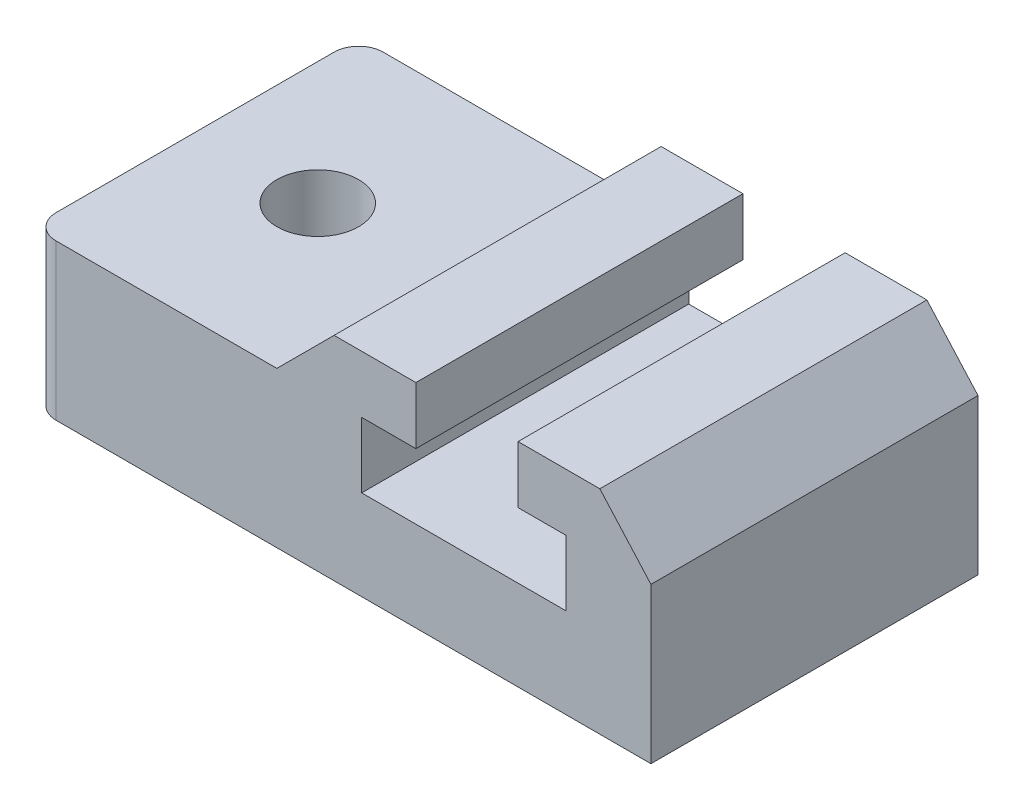
ISO-10303-21;
HEADER;
FILE_DESCRIPTION(('STEP AP214'),'2;1');
FILE_NAME('part.step','',(''),(''),'','','');
FILE_SCHEMA(('AUTOMOTIVE_DESIGN { 1 0 10303 214 1 1 1 1 }'));
ENDSEC;
DATA;
#1=APPLICATION_CONTEXT('core data for automotive mechanical design processes');
#2=APPLICATION_PROTOCOL_DEFINITION('international standard','automotive_design',2000,#1);
#3=PRODUCT_CONTEXT('',#1,'mechanical');
#4=PRODUCT('Part','Part','',(#3));
#5=PRODUCT_RELATED_PRODUCT_CATEGORY('part','',(#4));
#6=PRODUCT_DEFINITION_FORMATION('','',#4);
#7=PRODUCT_DEFINITION_CONTEXT('part definition',#1,'design');
#8=PRODUCT_DEFINITION('design','',#6,#7);
#9=PRODUCT_DEFINITION_SHAPE('','',#8);
#10=(LENGTH_UNIT() NAMED_UNIT(*) SI_UNIT(.MILLI.,.METRE.));
#11=(NAMED_UNIT(*) PLANE_ANGLE_UNIT() SI_UNIT($,.RADIAN.));
#12=(NAMED_UNIT(*) SI_UNIT($,.STERADIAN.) SOLID_ANGLE_UNIT());
#13=UNCERTAINTY_MEASURE_WITH_UNIT(LENGTH_MEASURE(1.E-05),#10,'distance_accuracy_value','');
#14=(GEOMETRIC_REPRESENTATION_CONTEXT(3) GLOBAL_UNCERTAINTY_ASSIGNED_CONTEXT((#13)) GLOBAL_UNIT_ASSIGNED_CONTEXT((#10,
#11,#12)) REPRESENTATION_CONTEXT('',''));
#15=CARTESIAN_POINT('',(0.,0.,0.));
#16=DIRECTION('',(0.,0.,1.));
#17=DIRECTION('',(1.,0.,0.));
#18=AXIS2_PLACEMENT_3D('',#15,#16,#17);
#19=CARTESIAN_POINT('',(0.,0.,80.));
#20=DIRECTION('',(0.,-1.,0.));
#21=DIRECTION('',(0.,0.,-1.));
#22=AXIS2_PLACEMENT_3D('',#19,#20,#21);
#23=PLANE('',#22);
#24=DIRECTION('',(0.,0.,1.));
#25=VECTOR('',#24,1.);
#26=CARTESIAN_POINT('',(-7.50000000000004,0.,6.));
#27=LINE('',#26,#25);
#28=CARTESIAN_POINT('',(-7.50000000000004,0.,61.0777233158545));
#29=VERTEX_POINT('',#28);
#30=CARTESIAN_POINT('',(-7.50000000000004,0.,74.));
#31=VERTEX_POINT('',#30);
#32=EDGE_CURVE('E308',#29,#31,#27,.T.);
#33=ORIENTED_EDGE('',*,*,#32,.F.);
#34=DIRECTION('',(-1.,0.,0.));
#35=VECTOR('',#34,1.);
#36=CARTESIAN_POINT('',(30.5,0.,61.0777233158545));
#37=LINE('',#36,#35);
#38=CARTESIAN_POINT('',(30.5,0.,61.0777233158545));
#39=VERTEX_POINT('',#38);
#40=EDGE_CURVE('E402',#39,#29,#37,.T.);
#41=ORIENTED_EDGE('',*,*,#40,.F.);
#42=DIRECTION('',(0.,0.,1.));
#43=VECTOR('',#42,1.);
#44=CARTESIAN_POINT('',(30.5,0.,0.));
#45=LINE('',#44,#43);
#46=CARTESIAN_POINT('',(30.5,0.,46.));
#47=VERTEX_POINT('',#46);
#48=EDGE_CURVE('E401',#47,#39,#45,.T.);
#49=ORIENTED_EDGE('',*,*,#48,.F.);
#50=CARTESIAN_POINT('',(22.5,0.,40.));
#51=DIRECTION('',(0.,1.,0.));
#52=DIRECTION('',(0.,0.,1.));
#53=AXIS2_PLACEMENT_3D('',#50,#51,#52);
#54=CIRCLE('',#53,10.);
#55=CARTESIAN_POINT('',(30.5,0.,34.));
#56=VERTEX_POINT('',#55);
#57=EDGE_CURVE('E290',#47,#56,#54,.T.);
#58=ORIENTED_EDGE('',*,*,#57,.T.);
#59=CARTESIAN_POINT('',(30.5,0.,18.2));
#60=VERTEX_POINT('',#59);
#61=EDGE_CURVE('E63',#60,#56,#45,.T.);
#62=ORIENTED_EDGE('',*,*,#61,.F.);
#63=DIRECTION('',(-1.,0.,0.));
#64=VECTOR('',#63,1.);
#65=CARTESIAN_POINT('',(30.5,0.,18.2));
#66=LINE('',#65,#64);
#67=CARTESIAN_POINT('',(-7.50000000000004,0.,18.2));
#68=VERTEX_POINT('',#67);
#69=EDGE_CURVE('E299',#60,#68,#66,.T.);
#70=ORIENTED_EDGE('',*,*,#69,.T.);
#71=CARTESIAN_POINT('',(-7.50000000000004,0.,6.));
#72=VERTEX_POINT('',#71);
#73=EDGE_CURVE('E306',#72,#68,#27,.T.);
#74=ORIENTED_EDGE('',*,*,#73,.F.);
#75=CARTESIAN_POINT('',(-1.50000000000004,0.,6.00000000000001));
#76=DIRECTION('',(0.,1.,0.));
#77=DIRECTION('',(0.,0.,1.));
#78=AXIS2_PLACEMENT_3D('',#75,#76,#77);
#79=CIRCLE('',#78,6.);
#80=CARTESIAN_POINT('',(-1.50000000000004,0.,0.));
#81=VERTEX_POINT('',#80);
#82=EDGE_CURVE('E304',#81,#72,#79,.T.);
#83=ORIENTED_EDGE('',*,*,#82,.F.);
#84=DIRECTION('',(-1.,0.,0.));
#85=VECTOR('',#84,1.);
#86=CARTESIAN_POINT('',(0.,0.,0.));
#87=LINE('',#86,#85);
#88=CARTESIAN_POINT('',(144.,0.,0.));
#89=VERTEX_POINT('',#88);
#90=EDGE_CURVE('E194',#89,#81,#87,.T.);
#91=ORIENTED_EDGE('',*,*,#90,.F.);
#92=DIRECTION('',(0.,0.,-1.));
#93=VECTOR('',#92,1.);
#94=CARTESIAN_POINT('',(144.,0.,80.));
#95=LINE('',#94,#93);
#96=CARTESIAN_POINT('',(144.,0.,80.));
#97=VERTEX_POINT('',#96);
#98=EDGE_CURVE('E251',#97,#89,#95,.T.);
#99=ORIENTED_EDGE('',*,*,#98,.F.);
#100=DIRECTION('',(-1.,0.,0.));
#101=VECTOR('',#100,1.);
#102=CARTESIAN_POINT('',(0.,0.,80.));
#103=LINE('',#102,#101);
#104=CARTESIAN_POINT('',(-1.50000000000004,0.,80.));
#105=VERTEX_POINT('',#104);
#106=EDGE_CURVE('E130',#97,#105,#103,.T.);
#107=ORIENTED_EDGE('',*,*,#106,.T.);
#108=CARTESIAN_POINT('',(-1.50000000000004,0.,74.));
#109=DIRECTION('',(0.,1.,0.));
#110=DIRECTION('',(0.,0.,1.));
#111=AXIS2_PLACEMENT_3D('',#108,#109,#110);
#112=CIRCLE('',#111,6.00000000000001);
#113=EDGE_CURVE('E313',#31,#105,#112,.T.);
#114=ORIENTED_EDGE('',*,*,#113,.F.);
#115=EDGE_LOOP('',(#33,#41,#49,#58,#62,#70,#74,#83,#91,#99,#107,#114));
#116=FACE_BOUND('',#115,.T.);
#117=ADVANCED_FACE('F50',(#116),#23,.T.);
#118=CARTESIAN_POINT('',(-7.50000000000004,0.,6.));
#119=DIRECTION('',(-1.,0.,0.));
#120=DIRECTION('',(0.,0.,1.));
#121=AXIS2_PLACEMENT_3D('',#118,#119,#120);
#122=PLANE('',#121);
#123=ORIENTED_EDGE('',*,*,#73,.T.);
#124=DIRECTION('',(0.,0.888265617173928,-0.459330157236188));
#125=VECTOR('',#124,1.);
#126=CARTESIAN_POINT('',(-7.50000000000004,7.42573077799279,14.3600876810915));
#127=LINE('',#126,#125);
#128=CARTESIAN_POINT('',(-7.50000000000004,11.9897349209895,12.));
#129=VERTEX_POINT('',#128);
#130=EDGE_CURVE('E398',#68,#129,#127,.T.);
#131=ORIENTED_EDGE('',*,*,#130,.T.);
#132=DIRECTION('',(0.,0.,1.));
#133=VECTOR('',#132,1.);
#134=CARTESIAN_POINT('',(-7.50000000000004,11.9897349209895,0.));
#135=LINE('',#134,#133);
#136=CARTESIAN_POINT('',(-7.50000000000004,11.9897349209895,68.));
#137=VERTEX_POINT('',#136);
#138=EDGE_CURVE('E404',#129,#137,#135,.T.);
#139=ORIENTED_EDGE('',*,*,#138,.T.);
#140=DIRECTION('',(0.,-0.866025403784439,-0.5));
#141=VECTOR('',#140,1.);
#142=CARTESIAN_POINT('',(-7.50000000000004,-26.4474299984236,45.8082924868908));
#143=LINE('',#142,#141);
#144=EDGE_CURVE('E412',#137,#29,#143,.T.);
#145=ORIENTED_EDGE('',*,*,#144,.T.);
#146=ORIENTED_EDGE('',*,*,#32,.T.);
#147=DIRECTION('',(0.,1.,0.));
#148=VECTOR('',#147,1.);
#149=CARTESIAN_POINT('',(-7.50000000000004,0.,74.));
#150=LINE('',#149,#148);
#151=CARTESIAN_POINT('',(-7.50000000000004,38.,74.));
#152=VERTEX_POINT('',#151);
#153=EDGE_CURVE('E191',#31,#152,#150,.T.);
#154=ORIENTED_EDGE('',*,*,#153,.T.);
#155=DIRECTION('',(0.,0.,1.));
#156=VECTOR('',#155,1.);
#157=CARTESIAN_POINT('',(-7.50000000000004,38.,6.));
#158=LINE('',#157,#156);
#159=CARTESIAN_POINT('',(-7.50000000000004,38.,6.));
#160=VERTEX_POINT('',#159);
#161=EDGE_CURVE('E294',#160,#152,#158,.T.);
#162=ORIENTED_EDGE('',*,*,#161,.F.);
#163=DIRECTION('',(0.,1.,0.));
#164=VECTOR('',#163,1.);
#165=CARTESIAN_POINT('',(-7.50000000000004,0.,6.));
#166=LINE('',#165,#164);
#167=EDGE_CURVE('E311',#72,#160,#166,.T.);
#168=ORIENTED_EDGE('',*,*,#167,.F.);
#169=EDGE_LOOP('',(#123,#131,#139,#145,#146,#154,#162,#168));
#170=FACE_BOUND('',#169,.T.);
#171=ADVANCED_FACE('F368',(#170),#122,.T.);
#172=CARTESIAN_POINT('',(22.5,0.,40.));
#173=DIRECTION('',(0.,1.,0.));
#174=DIRECTION('',(0.,0.,1.));
#175=AXIS2_PLACEMENT_3D('',#172,#173,#174);
#176=CYLINDRICAL_SURFACE('',#175,10.);
#177=CARTESIAN_POINT('',(22.5,38.,40.));
#178=DIRECTION('',(0.,1.,0.));
#179=DIRECTION('',(0.,0.,1.));
#180=AXIS2_PLACEMENT_3D('',#177,#178,#179);
#181=CIRCLE('',#180,10.);
#182=CARTESIAN_POINT('',(22.5,38.,50.));
#183=VERTEX_POINT('',#182);
#184=EDGE_CURVE('E292',#183,#183,#181,.T.);
#185=ORIENTED_EDGE('',*,*,#184,.T.);
#186=EDGE_LOOP('',(#185));
#187=FACE_BOUND('',#186,.T.);
#188=DIRECTION('',(0.,1.,0.));
#189=VECTOR('',#188,1.);
#190=CARTESIAN_POINT('',(30.5,0.,46.));
#191=LINE('',#190,#189);
#192=CARTESIAN_POINT('',(30.5,11.9897349209895,46.));
#193=VERTEX_POINT('',#192);
#194=EDGE_CURVE('E11',#193,#47,#191,.F.);
#195=ORIENTED_EDGE('',*,*,#194,.F.);
#196=CARTESIAN_POINT('',(22.5,11.9897349209895,40.));
#197=DIRECTION('',(0.,-1.,0.));
#198=DIRECTION('',(0.,0.,-1.));
#199=AXIS2_PLACEMENT_3D('',#196,#197,#198);
#200=CIRCLE('',#199,10.);
#201=CARTESIAN_POINT('',(30.5,11.9897349209895,34.));
#202=VERTEX_POINT('',#201);
#203=EDGE_CURVE('E53',#202,#193,#200,.F.);
#204=ORIENTED_EDGE('',*,*,#203,.F.);
#205=DIRECTION('',(0.,1.,0.));
#206=VECTOR('',#205,1.);
#207=CARTESIAN_POINT('',(30.5,0.,34.));
#208=LINE('',#207,#206);
#209=EDGE_CURVE('E254',#56,#202,#208,.T.);
#210=ORIENTED_EDGE('',*,*,#209,.F.);
#211=ORIENTED_EDGE('',*,*,#57,.F.);
#212=EDGE_LOOP('',(#195,#204,#210,#211));
#213=FACE_BOUND('',#212,.T.);
#214=ADVANCED_FACE('F284',(#187,#213),#176,.F.);
#215=CARTESIAN_POINT('',(144.,0.,80.));
#216=DIRECTION('',(1.,0.,0.));
#217=DIRECTION('',(0.,0.,-1.));
#218=AXIS2_PLACEMENT_3D('',#215,#216,#217);
#219=PLANE('',#218);
#220=DIRECTION('',(0.,-1.,0.));
#221=VECTOR('',#220,1.);
#222=CARTESIAN_POINT('',(144.,0.,0.));
#223=LINE('',#222,#221);
#224=CARTESIAN_POINT('',(144.,38.,0.));
#225=VERTEX_POINT('',#224);
#226=EDGE_CURVE('E197',#225,#89,#223,.T.);
#227=ORIENTED_EDGE('',*,*,#226,.F.);
#228=DIRECTION('',(0.,0.,-1.));
#229=VECTOR('',#228,1.);
#230=CARTESIAN_POINT('',(144.,38.,80.));
#231=LINE('',#230,#229);
#232=CARTESIAN_POINT('',(144.,38.,80.));
#233=VERTEX_POINT('',#232);
#234=EDGE_CURVE('E253',#233,#225,#231,.T.);
#235=ORIENTED_EDGE('',*,*,#234,.F.);
#236=DIRECTION('',(0.,-1.,0.));
#237=VECTOR('',#236,1.);
#238=CARTESIAN_POINT('',(144.,0.,80.));
#239=LINE('',#238,#237);
#240=EDGE_CURVE('E324',#233,#97,#239,.T.);
#241=ORIENTED_EDGE('',*,*,#240,.T.);
#242=ORIENTED_EDGE('',*,*,#98,.T.);
#243=EDGE_LOOP('',(#227,#235,#241,#242));
#244=FACE_BOUND('',#243,.T.);
#245=ADVANCED_FACE('F428',(#244),#219,.T.);
#246=CARTESIAN_POINT('',(99.0035486160397,88.3960255500355,80.));
#247=DIRECTION('',(0.745937661625914,0.666015769308853,0.));
#248=DIRECTION('',(-0.666015769308853,0.745937661625914,0.));
#249=AXIS2_PLACEMENT_3D('',#246,#247,#248);
#250=PLANE('',#249);
#251=DIRECTION('',(0.666015769308853,-0.745937661625914,0.));
#252=VECTOR('',#251,1.);
#253=CARTESIAN_POINT('',(99.0035486160397,88.3960255500355,0.));
#254=LINE('',#253,#252);
#255=CARTESIAN_POINT('',(131.5,52.,0.));
#256=VERTEX_POINT('',#255);
#257=EDGE_CURVE('E199',#256,#225,#254,.T.);
#258=ORIENTED_EDGE('',*,*,#257,.F.);
#259=DIRECTION('',(0.,0.,-1.));
#260=VECTOR('',#259,1.);
#261=CARTESIAN_POINT('',(131.5,52.,80.));
#262=LINE('',#261,#260);
#263=CARTESIAN_POINT('',(131.5,52.,80.));
#264=VERTEX_POINT('',#263);
#265=EDGE_CURVE('E246',#264,#256,#262,.T.);
#266=ORIENTED_EDGE('',*,*,#265,.F.);
#267=DIRECTION('',(0.666015769308853,-0.745937661625914,0.));
#268=VECTOR('',#267,1.);
#269=CARTESIAN_POINT('',(99.0035486160397,88.3960255500355,80.));
#270=LINE('',#269,#268);
#271=EDGE_CURVE('E327',#264,#233,#270,.T.);
#272=ORIENTED_EDGE('',*,*,#271,.T.);
#273=ORIENTED_EDGE('',*,*,#234,.T.);
#274=EDGE_LOOP('',(#258,#266,#272,#273));
#275=FACE_BOUND('',#274,.T.);
#276=ADVANCED_FACE('F435',(#275),#250,.T.);
#277=CARTESIAN_POINT('',(0.,52.,80.));
#278=DIRECTION('',(0.,1.,0.));
#279=DIRECTION('',(0.,0.,1.));
#280=AXIS2_PLACEMENT_3D('',#277,#278,#279);
#281=PLANE('',#280);
#282=DIRECTION('',(1.,0.,0.));
#283=VECTOR('',#282,1.);
#284=CARTESIAN_POINT('',(0.,52.,0.));
#285=LINE('',#284,#283);
#286=CARTESIAN_POINT('',(111.5,52.,0.));
#287=VERTEX_POINT('',#286);
#288=EDGE_CURVE('E201',#287,#256,#285,.T.);
#289=ORIENTED_EDGE('',*,*,#288,.F.);
#290=DIRECTION('',(0.,0.,-1.));
#291=VECTOR('',#290,1.);
#292=CARTESIAN_POINT('',(111.5,52.,80.));
#293=LINE('',#292,#291);
#294=CARTESIAN_POINT('',(111.5,52.,80.));
#295=VERTEX_POINT('',#294);
#296=EDGE_CURVE('E250',#295,#287,#293,.T.);
#297=ORIENTED_EDGE('',*,*,#296,.F.);
#298=DIRECTION('',(1.,0.,0.));
#299=VECTOR('',#298,1.);
#300=CARTESIAN_POINT('',(0.,52.,80.));
#301=LINE('',#300,#299);
#302=EDGE_CURVE('E332',#295,#264,#301,.T.);
#303=ORIENTED_EDGE('',*,*,#302,.T.);
#304=ORIENTED_EDGE('',*,*,#265,.T.);
#305=EDGE_LOOP('',(#289,#297,#303,#304));
#306=FACE_BOUND('',#305,.T.);
#307=ADVANCED_FACE('F436',(#306),#281,.T.);
#308=CARTESIAN_POINT('',(111.5,0.,80.));
#309=DIRECTION('',(1.,0.,0.));
#310=DIRECTION('',(0.,0.,-1.));
#311=AXIS2_PLACEMENT_3D('',#308,#309,#310);
#312=PLANE('',#311);
#313=DIRECTION('',(0.,-1.,0.));
#314=VECTOR('',#313,1.);
#315=CARTESIAN_POINT('',(111.5,0.,0.));
#316=LINE('',#315,#314);
#317=CARTESIAN_POINT('',(111.5,38.,0.));
#318=VERTEX_POINT('',#317);
#319=EDGE_CURVE('E206',#287,#318,#316,.T.);
#320=ORIENTED_EDGE('',*,*,#319,.T.);
#321=DIRECTION('',(0.,0.,-1.));
#322=VECTOR('',#321,1.);
#323=CARTESIAN_POINT('',(111.5,38.,80.));
#324=LINE('',#323,#322);
#325=CARTESIAN_POINT('',(111.5,38.,80.));
#326=VERTEX_POINT('',#325);
#327=EDGE_CURVE('E242',#326,#318,#324,.T.);
#328=ORIENTED_EDGE('',*,*,#327,.F.);
#329=DIRECTION('',(0.,-1.,0.));
#330=VECTOR('',#329,1.);
#331=CARTESIAN_POINT('',(111.5,0.,80.));
#332=LINE('',#331,#330);
#333=EDGE_CURVE('E331',#295,#326,#332,.T.);
#334=ORIENTED_EDGE('',*,*,#333,.F.);
#335=ORIENTED_EDGE('',*,*,#296,.T.);
#336=EDGE_LOOP('',(#320,#328,#334,#335));
#337=FACE_BOUND('',#336,.T.);
#338=ADVANCED_FACE('F442',(#337),#312,.F.);
#339=CARTESIAN_POINT('',(0.,38.,80.));
#340=DIRECTION('',(0.,1.,0.));
#341=DIRECTION('',(0.,0.,1.));
#342=AXIS2_PLACEMENT_3D('',#339,#340,#341);
#343=PLANE('',#342);
#344=DIRECTION('',(1.,0.,0.));
#345=VECTOR('',#344,1.);
#346=CARTESIAN_POINT('',(0.,38.,0.));
#347=LINE('',#346,#345);
#348=CARTESIAN_POINT('',(123.25,38.,0.));
#349=VERTEX_POINT('',#348);
#350=EDGE_CURVE('E208',#318,#349,#347,.T.);
#351=ORIENTED_EDGE('',*,*,#350,.T.);
#352=DIRECTION('',(0.,0.,-1.));
#353=VECTOR('',#352,1.);
#354=CARTESIAN_POINT('',(123.25,38.,80.));
#355=LINE('',#354,#353);
#356=CARTESIAN_POINT('',(123.25,38.,80.));
#357=VERTEX_POINT('',#356);
#358=EDGE_CURVE('E243',#357,#349,#355,.T.);
#359=ORIENTED_EDGE('',*,*,#358,.F.);
#360=DIRECTION('',(1.,0.,0.));
#361=VECTOR('',#360,1.);
#362=CARTESIAN_POINT('',(0.,38.,80.));
#363=LINE('',#362,#361);
#364=EDGE_CURVE('E338',#326,#357,#363,.T.);
#365=ORIENTED_EDGE('',*,*,#364,.F.);
#366=ORIENTED_EDGE('',*,*,#327,.T.);
#367=EDGE_LOOP('',(#351,#359,#365,#366));
#368=FACE_BOUND('',#367,.T.);
#369=ADVANCED_FACE('F450',(#368),#343,.F.);
#370=CARTESIAN_POINT('',(123.25,0.,80.));
#371=DIRECTION('',(1.,0.,0.));
#372=DIRECTION('',(0.,0.,-1.));
#373=AXIS2_PLACEMENT_3D('',#370,#371,#372);
#374=PLANE('',#373);
#375=DIRECTION('',(0.,-1.,0.));
#376=VECTOR('',#375,1.);
#377=CARTESIAN_POINT('',(123.25,0.,0.));
#378=LINE('',#377,#376);
#379=CARTESIAN_POINT('',(123.25,22.,0.));
#380=VERTEX_POINT('',#379);
#381=EDGE_CURVE('E209',#349,#380,#378,.T.);
#382=ORIENTED_EDGE('',*,*,#381,.T.);
#383=DIRECTION('',(0.,0.,-1.));
#384=VECTOR('',#383,1.);
#385=CARTESIAN_POINT('',(123.25,22.,80.));
#386=LINE('',#385,#384);
#387=CARTESIAN_POINT('',(123.25,22.,80.));
#388=VERTEX_POINT('',#387);
#389=EDGE_CURVE('E236',#388,#380,#386,.T.);
#390=ORIENTED_EDGE('',*,*,#389,.F.);
#391=DIRECTION('',(0.,-1.,0.));
#392=VECTOR('',#391,1.);
#393=CARTESIAN_POINT('',(123.25,0.,80.));
#394=LINE('',#393,#392);
#395=EDGE_CURVE('E336',#357,#388,#394,.T.);
#396=ORIENTED_EDGE('',*,*,#395,.F.);
#397=ORIENTED_EDGE('',*,*,#358,.T.);
#398=EDGE_LOOP('',(#382,#390,#396,#397));
#399=FACE_BOUND('',#398,.T.);
#400=ADVANCED_FACE('F452',(#399),#374,.F.);
#401=CARTESIAN_POINT('',(0.,22.,80.));
#402=DIRECTION('',(0.,-1.,0.));
#403=DIRECTION('',(0.,0.,-1.));
#404=AXIS2_PLACEMENT_3D('',#401,#402,#403);
#405=PLANE('',#404);
#406=DIRECTION('',(-1.,0.,0.));
#407=VECTOR('',#406,1.);
#408=CARTESIAN_POINT('',(0.,22.,0.));
#409=LINE('',#408,#407);
#410=CARTESIAN_POINT('',(73.25,22.,0.));
#411=VERTEX_POINT('',#410);
#412=EDGE_CURVE('E215',#380,#411,#409,.T.);
#413=ORIENTED_EDGE('',*,*,#412,.T.);
#414=DIRECTION('',(0.,0.,-1.));
#415=VECTOR('',#414,1.);
#416=CARTESIAN_POINT('',(73.25,22.,80.));
#417=LINE('',#416,#415);
#418=CARTESIAN_POINT('',(73.25,22.,80.));
#419=VERTEX_POINT('',#418);
#420=EDGE_CURVE('E233',#419,#411,#417,.T.);
#421=ORIENTED_EDGE('',*,*,#420,.F.);
#422=DIRECTION('',(-1.,0.,0.));
#423=VECTOR('',#422,1.);
#424=CARTESIAN_POINT('',(0.,22.,80.));
#425=LINE('',#424,#423);
#426=EDGE_CURVE('E339',#388,#419,#425,.T.);
#427=ORIENTED_EDGE('',*,*,#426,.F.);
#428=ORIENTED_EDGE('',*,*,#389,.T.);
#429=EDGE_LOOP('',(#413,#421,#427,#428));
#430=FACE_BOUND('',#429,.T.);
#431=ADVANCED_FACE('F457',(#430),#405,.F.);
#432=CARTESIAN_POINT('',(73.25,0.,80.));
#433=DIRECTION('',(-1.,0.,0.));
#434=DIRECTION('',(0.,0.,1.));
#435=AXIS2_PLACEMENT_3D('',#432,#433,#434);
#436=PLANE('',#435);
#437=DIRECTION('',(0.,1.,0.));
#438=VECTOR('',#437,1.);
#439=CARTESIAN_POINT('',(73.25,0.,0.));
#440=LINE('',#439,#438);
#441=CARTESIAN_POINT('',(73.25,38.,0.));
#442=VERTEX_POINT('',#441);
#443=EDGE_CURVE('E212',#411,#442,#440,.T.);
#444=ORIENTED_EDGE('',*,*,#443,.T.);
#445=DIRECTION('',(0.,0.,-1.));
#446=VECTOR('',#445,1.);
#447=CARTESIAN_POINT('',(73.25,38.,80.));
#448=LINE('',#447,#446);
#449=CARTESIAN_POINT('',(73.25,38.,80.));
#450=VERTEX_POINT('',#449);
#451=EDGE_CURVE('E234',#450,#442,#448,.T.);
#452=ORIENTED_EDGE('',*,*,#451,.F.);
#453=DIRECTION('',(0.,1.,0.));
#454=VECTOR('',#453,1.);
#455=CARTESIAN_POINT('',(73.25,0.,80.));
#456=LINE('',#455,#454);
#457=EDGE_CURVE('E345',#419,#450,#456,.T.);
#458=ORIENTED_EDGE('',*,*,#457,.F.);
#459=ORIENTED_EDGE('',*,*,#420,.T.);
#460=EDGE_LOOP('',(#444,#452,#458,#459));
#461=FACE_BOUND('',#460,.T.);
#462=ADVANCED_FACE('F458',(#461),#436,.F.);
#463=CARTESIAN_POINT('',(0.,38.,80.));
#464=DIRECTION('',(0.,-1.,0.));
#465=DIRECTION('',(0.,0.,-1.));
#466=AXIS2_PLACEMENT_3D('',#463,#464,#465);
#467=PLANE('',#466);
#468=DIRECTION('',(-1.,0.,0.));
#469=VECTOR('',#468,1.);
#470=CARTESIAN_POINT('',(0.,38.,0.));
#471=LINE('',#470,#469);
#472=CARTESIAN_POINT('',(86.5,38.,0.));
#473=VERTEX_POINT('',#472);
#474=EDGE_CURVE('E220',#473,#442,#471,.T.);
#475=ORIENTED_EDGE('',*,*,#474,.F.);
#476=DIRECTION('',(0.,0.,-1.));
#477=VECTOR('',#476,1.);
#478=CARTESIAN_POINT('',(86.5,38.,80.));
#479=LINE('',#478,#477);
#480=CARTESIAN_POINT('',(86.5,38.,80.));
#481=VERTEX_POINT('',#480);
#482=EDGE_CURVE('E232',#481,#473,#479,.T.);
#483=ORIENTED_EDGE('',*,*,#482,.F.);
#484=DIRECTION('',(-1.,0.,0.));
#485=VECTOR('',#484,1.);
#486=CARTESIAN_POINT('',(0.,38.,80.));
#487=LINE('',#486,#485);
#488=EDGE_CURVE('E341',#481,#450,#487,.T.);
#489=ORIENTED_EDGE('',*,*,#488,.T.);
#490=ORIENTED_EDGE('',*,*,#451,.T.);
#491=EDGE_LOOP('',(#475,#483,#489,#490));
#492=FACE_BOUND('',#491,.T.);
#493=ADVANCED_FACE('F461',(#492),#467,.T.);
#494=CARTESIAN_POINT('',(86.5,0.,80.));
#495=DIRECTION('',(1.,0.,0.));
#496=DIRECTION('',(0.,0.,-1.));
#497=AXIS2_PLACEMENT_3D('',#494,#495,#496);
#498=PLANE('',#497);
#499=DIRECTION('',(0.,-1.,0.));
#500=VECTOR('',#499,1.);
#501=CARTESIAN_POINT('',(86.5,0.,0.));
#502=LINE('',#501,#500);
#503=CARTESIAN_POINT('',(86.5,52.,0.));
#504=VERTEX_POINT('',#503);
#505=EDGE_CURVE('E219',#504,#473,#502,.T.);
#506=ORIENTED_EDGE('',*,*,#505,.F.);
#507=DIRECTION('',(0.,0.,-1.));
#508=VECTOR('',#507,1.);
#509=CARTESIAN_POINT('',(86.5,52.,80.));
#510=LINE('',#509,#508);
#511=CARTESIAN_POINT('',(86.5,52.,80.));
#512=VERTEX_POINT('',#511);
#513=EDGE_CURVE('E181',#512,#504,#510,.T.);
#514=ORIENTED_EDGE('',*,*,#513,.F.);
#515=DIRECTION('',(0.,-1.,0.));
#516=VECTOR('',#515,1.);
#517=CARTESIAN_POINT('',(86.5,0.,80.));
#518=LINE('',#517,#516);
#519=EDGE_CURVE('E175',#512,#481,#518,.T.);
#520=ORIENTED_EDGE('',*,*,#519,.T.);
#521=ORIENTED_EDGE('',*,*,#482,.T.);
#522=EDGE_LOOP('',(#506,#514,#520,#521));
#523=FACE_BOUND('',#522,.T.);
#524=ADVANCED_FACE('F346',(#523),#498,.T.);
#525=CARTESIAN_POINT('',(0.,52.,80.));
#526=DIRECTION('',(0.,-1.,0.));
#527=DIRECTION('',(0.,0.,-1.));
#528=AXIS2_PLACEMENT_3D('',#525,#526,#527);
#529=PLANE('',#528);
#530=DIRECTION('',(-1.,0.,0.));
#531=VECTOR('',#530,1.);
#532=CARTESIAN_POINT('',(0.,52.,0.));
#533=LINE('',#532,#531);
#534=CARTESIAN_POINT('',(66.5,52.,0.));
#535=VERTEX_POINT('',#534);
#536=EDGE_CURVE('E176',#504,#535,#533,.T.);
#537=ORIENTED_EDGE('',*,*,#536,.T.);
#538=DIRECTION('',(0.,0.,-1.));
#539=VECTOR('',#538,1.);
#540=CARTESIAN_POINT('',(66.5,52.,80.));
#541=LINE('',#540,#539);
#542=CARTESIAN_POINT('',(66.5,52.,80.));
#543=VERTEX_POINT('',#542);
#544=EDGE_CURVE('E177',#543,#535,#541,.T.);
#545=ORIENTED_EDGE('',*,*,#544,.F.);
#546=DIRECTION('',(-1.,0.,0.));
#547=VECTOR('',#546,1.);
#548=CARTESIAN_POINT('',(0.,52.,80.));
#549=LINE('',#548,#547);
#550=EDGE_CURVE('E164',#512,#543,#549,.T.);
#551=ORIENTED_EDGE('',*,*,#550,.F.);
#552=ORIENTED_EDGE('',*,*,#513,.T.);
#553=EDGE_LOOP('',(#537,#545,#551,#552));
#554=FACE_BOUND('',#553,.T.);
#555=ADVANCED_FACE('F180',(#554),#529,.F.);
#556=CARTESIAN_POINT('',(7.24999999999998,-7.24999999999998,80.));
#557=DIRECTION('',(-0.707106781186548,0.707106781186548,0.));
#558=DIRECTION('',(-0.707106781186548,-0.707106781186548,0.));
#559=AXIS2_PLACEMENT_3D('',#556,#557,#558);
#560=PLANE('',#559);
#561=DIRECTION('',(0.707106781186548,0.707106781186548,0.));
#562=VECTOR('',#561,1.);
#563=CARTESIAN_POINT('',(7.24999999999998,-7.24999999999998,0.));
#564=LINE('',#563,#562);
#565=CARTESIAN_POINT('',(52.5,38.,0.));
#566=VERTEX_POINT('',#565);
#567=EDGE_CURVE('E221',#566,#535,#564,.T.);
#568=ORIENTED_EDGE('',*,*,#567,.F.);
#569=DIRECTION('',(0.,0.,-1.));
#570=VECTOR('',#569,1.);
#571=CARTESIAN_POINT('',(52.5,38.,80.));
#572=LINE('',#571,#570);
#573=CARTESIAN_POINT('',(52.5,38.,80.));
#574=VERTEX_POINT('',#573);
#575=EDGE_CURVE('E116',#574,#566,#572,.T.);
#576=ORIENTED_EDGE('',*,*,#575,.F.);
#577=DIRECTION('',(0.707106781186548,0.707106781186548,0.));
#578=VECTOR('',#577,1.);
#579=CARTESIAN_POINT('',(7.24999999999998,-7.24999999999998,80.));
#580=LINE('',#579,#578);
#581=EDGE_CURVE('E166',#574,#543,#580,.T.);
#582=ORIENTED_EDGE('',*,*,#581,.T.);
#583=ORIENTED_EDGE('',*,*,#544,.T.);
#584=EDGE_LOOP('',(#568,#576,#582,#583));
#585=FACE_BOUND('',#584,.T.);
#586=ADVANCED_FACE('F183',(#585),#560,.T.);
#587=CARTESIAN_POINT('',(0.,38.,80.));
#588=DIRECTION('',(0.,-1.,0.));
#589=DIRECTION('',(0.,0.,-1.));
#590=AXIS2_PLACEMENT_3D('',#587,#588,#589);
#591=PLANE('',#590);
#592=ORIENTED_EDGE('',*,*,#184,.F.);
#593=EDGE_LOOP('',(#592));
#594=FACE_BOUND('',#593,.T.);
#595=DIRECTION('',(-1.,0.,0.));
#596=VECTOR('',#595,1.);
#597=CARTESIAN_POINT('',(0.,38.,0.));
#598=LINE('',#597,#596);
#599=CARTESIAN_POINT('',(-1.50000000000004,38.,0.));
#600=VERTEX_POINT('',#599);
#601=EDGE_CURVE('E228',#566,#600,#598,.T.);
#602=ORIENTED_EDGE('',*,*,#601,.T.);
#603=CARTESIAN_POINT('',(-1.50000000000004,38.,6.00000000000001));
#604=DIRECTION('',(0.,1.,0.));
#605=DIRECTION('',(0.,0.,1.));
#606=AXIS2_PLACEMENT_3D('',#603,#604,#605);
#607=CIRCLE('',#606,6.);
#608=EDGE_CURVE('E288',#600,#160,#607,.T.);
#609=ORIENTED_EDGE('',*,*,#608,.T.);
#610=ORIENTED_EDGE('',*,*,#161,.T.);
#611=CARTESIAN_POINT('',(-1.50000000000004,38.,74.));
#612=DIRECTION('',(0.,1.,0.));
#613=DIRECTION('',(0.,0.,1.));
#614=AXIS2_PLACEMENT_3D('',#611,#612,#613);
#615=CIRCLE('',#614,6.00000000000001);
#616=CARTESIAN_POINT('',(-1.50000000000004,38.,80.));
#617=VERTEX_POINT('',#616);
#618=EDGE_CURVE('E307',#152,#617,#615,.T.);
#619=ORIENTED_EDGE('',*,*,#618,.T.);
#620=DIRECTION('',(-1.,0.,0.));
#621=VECTOR('',#620,1.);
#622=CARTESIAN_POINT('',(0.,38.,80.));
#623=LINE('',#622,#621);
#624=EDGE_CURVE('E68',#574,#617,#623,.T.);
#625=ORIENTED_EDGE('',*,*,#624,.F.);
#626=ORIENTED_EDGE('',*,*,#575,.T.);
#627=EDGE_LOOP('',(#602,#609,#610,#619,#625,#626));
#628=FACE_BOUND('',#627,.T.);
#629=ADVANCED_FACE('F352',(#594,#628),#591,.F.);
#630=CARTESIAN_POINT('',(0.,0.,80.));
#631=DIRECTION('',(0.,0.,1.));
#632=DIRECTION('',(1.,0.,0.));
#633=AXIS2_PLACEMENT_3D('',#630,#631,#632);
#634=PLANE('',#633);
#635=DIRECTION('',(0.,-1.,0.));
#636=VECTOR('',#635,1.);
#637=CARTESIAN_POINT('',(-1.50000000000004,0.,80.));
#638=LINE('',#637,#636);
#639=EDGE_CURVE('E226',#617,#105,#638,.T.);
#640=ORIENTED_EDGE('',*,*,#639,.T.);
#641=ORIENTED_EDGE('',*,*,#106,.F.);
#642=ORIENTED_EDGE('',*,*,#240,.F.);
#643=ORIENTED_EDGE('',*,*,#271,.F.);
#644=ORIENTED_EDGE('',*,*,#302,.F.);
#645=ORIENTED_EDGE('',*,*,#333,.T.);
#646=ORIENTED_EDGE('',*,*,#364,.T.);
#647=ORIENTED_EDGE('',*,*,#395,.T.);
#648=ORIENTED_EDGE('',*,*,#426,.T.);
#649=ORIENTED_EDGE('',*,*,#457,.T.);
#650=ORIENTED_EDGE('',*,*,#488,.F.);
#651=ORIENTED_EDGE('',*,*,#519,.F.);
#652=ORIENTED_EDGE('',*,*,#550,.T.);
#653=ORIENTED_EDGE('',*,*,#581,.F.);
#654=ORIENTED_EDGE('',*,*,#624,.T.);
#655=EDGE_LOOP('',(#640,#641,#642,#643,#644,#645,#646,#647,#648,#649,#650,#651,#652,#653,#654));
#656=FACE_BOUND('',#655,.T.);
#657=ADVANCED_FACE('F170',(#656),#634,.T.);
#658=CARTESIAN_POINT('',(0.,0.,0.));
#659=DIRECTION('',(0.,0.,1.));
#660=DIRECTION('',(1.,0.,0.));
#661=AXIS2_PLACEMENT_3D('',#658,#659,#660);
#662=PLANE('',#661);
#663=ORIENTED_EDGE('',*,*,#90,.T.);
#664=DIRECTION('',(0.,-1.,0.));
#665=VECTOR('',#664,1.);
#666=CARTESIAN_POINT('',(-1.50000000000004,0.,0.));
#667=LINE('',#666,#665);
#668=EDGE_CURVE('E189',#600,#81,#667,.T.);
#669=ORIENTED_EDGE('',*,*,#668,.F.);
#670=ORIENTED_EDGE('',*,*,#601,.F.);
#671=ORIENTED_EDGE('',*,*,#567,.T.);
#672=ORIENTED_EDGE('',*,*,#536,.F.);
#673=ORIENTED_EDGE('',*,*,#505,.T.);
#674=ORIENTED_EDGE('',*,*,#474,.T.);
#675=ORIENTED_EDGE('',*,*,#443,.F.);
#676=ORIENTED_EDGE('',*,*,#412,.F.);
#677=ORIENTED_EDGE('',*,*,#381,.F.);
#678=ORIENTED_EDGE('',*,*,#350,.F.);
#679=ORIENTED_EDGE('',*,*,#319,.F.);
#680=ORIENTED_EDGE('',*,*,#288,.T.);
#681=ORIENTED_EDGE('',*,*,#257,.T.);
#682=ORIENTED_EDGE('',*,*,#226,.T.);
#683=EDGE_LOOP('',(#663,#669,#670,#671,#672,#673,#674,#675,#676,#677,#678,#679,#680,#681,#682));
#684=FACE_BOUND('',#683,.T.);
#685=ADVANCED_FACE('F353',(#684),#662,.F.);
#686=CARTESIAN_POINT('',(-1.50000000000004,0.,6.00000000000001));
#687=DIRECTION('',(0.,1.,0.));
#688=DIRECTION('',(0.,0.,1.));
#689=AXIS2_PLACEMENT_3D('',#686,#687,#688);
#690=CYLINDRICAL_SURFACE('',#689,6.);
#691=ORIENTED_EDGE('',*,*,#608,.F.);
#692=ORIENTED_EDGE('',*,*,#668,.T.);
#693=ORIENTED_EDGE('',*,*,#82,.T.);
#694=ORIENTED_EDGE('',*,*,#167,.T.);
#695=EDGE_LOOP('',(#691,#692,#693,#694));
#696=FACE_BOUND('',#695,.T.);
#697=ADVANCED_FACE('F356',(#696),#690,.T.);
#698=CARTESIAN_POINT('',(-1.50000000000004,0.,74.));
#699=DIRECTION('',(0.,1.,0.));
#700=DIRECTION('',(0.,0.,1.));
#701=AXIS2_PLACEMENT_3D('',#698,#699,#700);
#702=CYLINDRICAL_SURFACE('',#701,6.00000000000001);
#703=ORIENTED_EDGE('',*,*,#618,.F.);
#704=ORIENTED_EDGE('',*,*,#153,.F.);
#705=ORIENTED_EDGE('',*,*,#113,.T.);
#706=ORIENTED_EDGE('',*,*,#639,.F.);
#707=EDGE_LOOP('',(#703,#704,#705,#706));
#708=FACE_BOUND('',#707,.T.);
#709=ADVANCED_FACE('F421',(#708),#702,.T.);
#710=CARTESIAN_POINT('',(30.5,11.9897349209895,0.));
#711=DIRECTION('',(0.,-1.,0.));
#712=DIRECTION('',(0.,0.,-1.));
#713=AXIS2_PLACEMENT_3D('',#710,#711,#712);
#714=PLANE('',#713);
#715=ORIENTED_EDGE('',*,*,#203,.T.);
#716=DIRECTION('',(0.,0.,1.));
#717=VECTOR('',#716,1.);
#718=CARTESIAN_POINT('',(30.5,11.9897349209895,0.));
#719=LINE('',#718,#717);
#720=CARTESIAN_POINT('',(30.5,11.9897349209895,68.));
#721=VERTEX_POINT('',#720);
#722=EDGE_CURVE('E266',#193,#721,#719,.T.);
#723=ORIENTED_EDGE('',*,*,#722,.T.);
#724=DIRECTION('',(-1.,0.,0.));
#725=VECTOR('',#724,1.);
#726=CARTESIAN_POINT('',(30.5,11.9897349209895,68.));
#727=LINE('',#726,#725);
#728=EDGE_CURVE('E417',#721,#137,#727,.T.);
#729=ORIENTED_EDGE('',*,*,#728,.T.);
#730=ORIENTED_EDGE('',*,*,#138,.F.);
#731=DIRECTION('',(-1.,0.,0.));
#732=VECTOR('',#731,1.);
#733=CARTESIAN_POINT('',(30.5,11.9897349209895,12.));
#734=LINE('',#733,#732);
#735=CARTESIAN_POINT('',(30.5,11.9897349209895,12.));
#736=VERTEX_POINT('',#735);
#737=EDGE_CURVE('E300',#736,#129,#734,.T.);
#738=ORIENTED_EDGE('',*,*,#737,.F.);
#739=EDGE_CURVE('E271',#736,#202,#719,.T.);
#740=ORIENTED_EDGE('',*,*,#739,.T.);
#741=EDGE_LOOP('',(#715,#723,#729,#730,#738,#740));
#742=FACE_BOUND('',#741,.T.);
#743=ADVANCED_FACE('F263',(#742),#714,.T.);
#744=CARTESIAN_POINT('',(30.5,0.,0.));
#745=DIRECTION('',(-1.,0.,0.));
#746=DIRECTION('',(0.,0.,1.));
#747=AXIS2_PLACEMENT_3D('',#744,#745,#746);
#748=PLANE('',#747);
#749=ORIENTED_EDGE('',*,*,#194,.T.);
#750=ORIENTED_EDGE('',*,*,#48,.T.);
#751=DIRECTION('',(0.,-0.866025403784439,-0.5));
#752=VECTOR('',#751,1.);
#753=CARTESIAN_POINT('',(30.5,-26.4474299984236,45.8082924868908));
#754=LINE('',#753,#752);
#755=EDGE_CURVE('E285',#721,#39,#754,.T.);
#756=ORIENTED_EDGE('',*,*,#755,.F.);
#757=ORIENTED_EDGE('',*,*,#722,.F.);
#758=EDGE_LOOP('',(#749,#750,#756,#757));
#759=FACE_BOUND('',#758,.T.);
#760=ADVANCED_FACE('F279',(#759),#748,.T.);
#761=ORIENTED_EDGE('',*,*,#209,.T.);
#762=ORIENTED_EDGE('',*,*,#739,.F.);
#763=DIRECTION('',(0.,0.888265617173928,-0.459330157236188));
#764=VECTOR('',#763,1.);
#765=CARTESIAN_POINT('',(30.5,7.42573077799279,14.3600876810915));
#766=LINE('',#765,#764);
#767=EDGE_CURVE('E399',#60,#736,#766,.T.);
#768=ORIENTED_EDGE('',*,*,#767,.F.);
#769=ORIENTED_EDGE('',*,*,#61,.T.);
#770=EDGE_LOOP('',(#761,#762,#768,#769));
#771=FACE_BOUND('',#770,.T.);
#772=ADVANCED_FACE('F405',(#771),#748,.T.);
#773=CARTESIAN_POINT('',(30.5,7.42573077799279,14.3600876810915));
#774=DIRECTION('',(0.,0.459330157236188,0.888265617173928));
#775=DIRECTION('',(0.,-0.888265617173928,0.459330157236188));
#776=AXIS2_PLACEMENT_3D('',#773,#774,#775);
#777=PLANE('',#776);
#778=ORIENTED_EDGE('',*,*,#130,.F.);
#779=ORIENTED_EDGE('',*,*,#69,.F.);
#780=ORIENTED_EDGE('',*,*,#767,.T.);
#781=ORIENTED_EDGE('',*,*,#737,.T.);
#782=EDGE_LOOP('',(#778,#779,#780,#781));
#783=FACE_BOUND('',#782,.T.);
#784=ADVANCED_FACE('F397',(#783),#777,.T.);
#785=CARTESIAN_POINT('',(30.5,-26.4474299984236,45.8082924868908));
#786=DIRECTION('',(0.,0.5,-0.866025403784439));
#787=DIRECTION('',(0.,0.866025403784439,0.5));
#788=AXIS2_PLACEMENT_3D('',#785,#786,#787);
#789=PLANE('',#788);
#790=ORIENTED_EDGE('',*,*,#144,.F.);
#791=ORIENTED_EDGE('',*,*,#728,.F.);
#792=ORIENTED_EDGE('',*,*,#755,.T.);
#793=ORIENTED_EDGE('',*,*,#40,.T.);
#794=EDGE_LOOP('',(#790,#791,#792,#793));
#795=FACE_BOUND('',#794,.T.);
#796=ADVANCED_FACE('F423',(#795),#789,.T.);
#797=CLOSED_SHELL('',(#117,#171,#214,#245,#276,#307,#338,#369,#400,#431,#462,#493,#524,#555,
#586,#629,#657,#685,#697,#709,#743,#760,#772,#784,#796));
#798=MANIFOLD_SOLID_BREP('B2',#797);
#799=ADVANCED_BREP_SHAPE_REPRESENTATION('',(#18,#798),#14);
#800=SHAPE_DEFINITION_REPRESENTATION(#9,#799);
ENDSEC;
END-ISO-10303-21;
